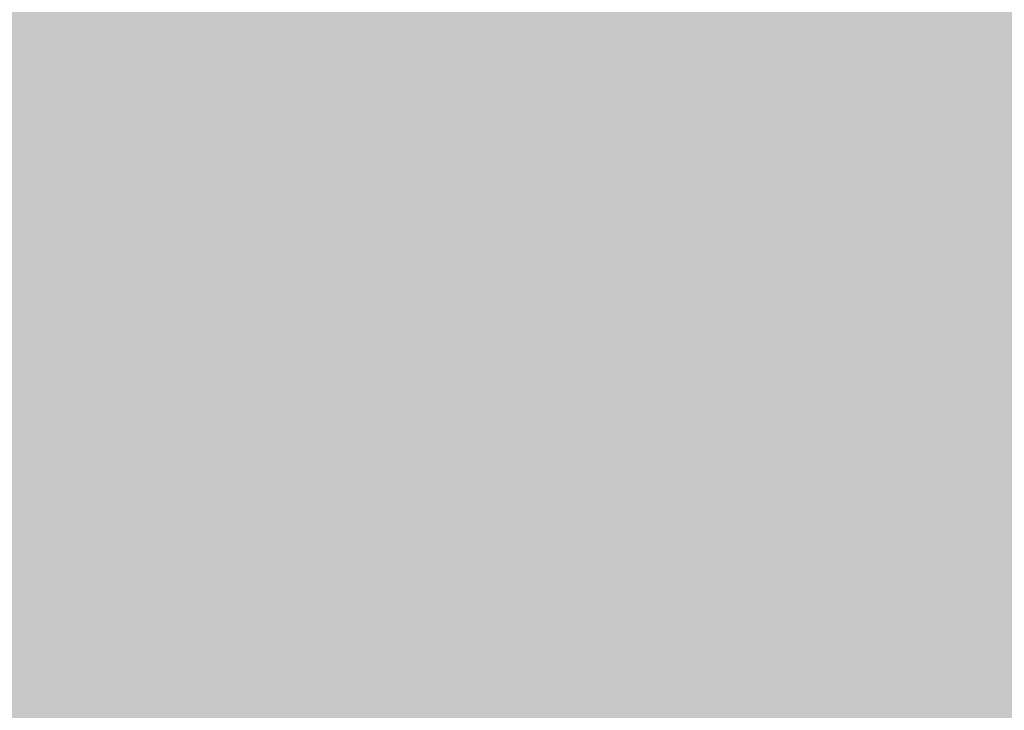
# Model space of a CAD drawing. Units: inches. Extents: x 2091 to 2899, y 967 to 2217.
# Tile 179 of 256: x 2203.151632 to 2203.161218, y 1152.253784 to 1152.260509. Entities that reach past the tile are written whole.
import ezdxf

# ---------------------------------------------------------------- set-up
doc = ezdxf.new("R2010")
doc.units = ezdxf.units.IN
doc.layers.add('A-WALL-PATT', color=141, linetype='Continuous', lineweight=13, true_color=0xadddf7)

msp = doc.modelspace()

# ---------------------------------------------------------------- hatches: boundary and pattern name
at = {"layer": 'A-WALL-PATT'}
h = msp.add_hatch(color=256, dxfattribs=at)
h.dxf.hatch_style = 1
h.paths.add_polyline_path([(2803.1436027, 2050.9190588), (2203.1436027, 2050.9190588), (2203.1436027, 1090.9190588), (2803.1436027, 1090.9190588)])
h.paths.add_polyline_path([(2635.7988501, 1147.5404649), (2674.5240524, 1147.5404649, 0.376086), (2678.5296653, 1152.8802017), (2678.5296653, 1159.5564734, 0.333335), (2674.524319, 1163.561846), (2674.524319, 1163.5618504), (2674.524319, 1192.9343904), (2635.8059707, 1192.9343904), (2597.0876225, 1192.9343904), (2597.0876225, 1163.561846, 0.333335), (2593.0822761, 1159.5564734), (2593.0822761, 1152.8802017, 0.376086), (2597.087889, 1147.5404649)], flags=0)
h.paths.add_polyline_path([(2436.0104329, 1278.2407784, 0.000483), (2435.9526433, 1278.215027, -0.001328), (2435.9356253, 1278.1116934, -0.001711), (2436.1164401, 1278.0407583, 0.002185)], flags=0)
h.paths.add_polyline_path([(2794.1436027, 1143.4190588), (2794.1436027, 1347.4190588), (2543.3701706, 1347.4190588), (2543.3701706, 1351.9190588), (2794.1436027, 1351.9190588), (2794.1436027, 1392.7135549), (2793.9473982, 1392.7135549), (2793.9473982, 1473.5368999), (2794.1436027, 1473.5368999), (2794.1436027, 1531.9190588), (2650.1436027, 1531.9190588), (2650.1436027, 1536.4190588), (2794.1436027, 1536.4190588), (2794.1436027, 1692.4190588), (2609.3756095, 1692.4190588), (2609.3756095, 1644.4190588), (2604.8756095, 1644.4190588), (2604.8756095, 1744.9190588), (2609.3756095, 1744.9190588), (2609.3756095, 1696.9190588), (2794.1436027, 1696.9190588), (2794.1436027, 1780.9190588), (2609.6436027, 1780.9190588), (2493.8756095, 1780.9190588), (2493.8756095, 1785.4190588), (2609.6436027, 1785.4190588), (2794.1436027, 1785.4190588), (2794.1436027, 1847.9388214), (2793.9512217, 1847.9388214), (2793.9512217, 1928.7621663), (2794.1436027, 1928.7621663), (2794.1436027, 1941.4190588), (2614.1436027, 1941.4190588), (2614.1436027, 1821.4190588), (2609.6436027, 1821.4190588), (2609.6436027, 1941.4190588), (2392.1436027, 1941.4190588), (2392.1436027, 1819.9190588), (2387.6436027, 1819.9190588), (2387.6436027, 1941.4190588), (2212.1436027, 1941.4190588), (2212.1436027, 1783.9190588), (2392.1436027, 1783.9190588), (2392.1436027, 1780.9190588), (2212.1436027, 1780.9190588), (2212.1436027, 1629.4190588), (2387.6436027, 1629.4190588), (2387.6436027, 1744.9190588), (2392.1436027, 1744.9190588), (2392.1436027, 1627.9190588), (2317.1436027, 1627.9190588), (2317.1436027, 1551.4190588), (2317.1436027, 1536.4190588), (2459.3835909, 1536.4190588), (2459.3835909, 1602.3964802), (2463.8835909, 1602.3964802), (2463.8835909, 1531.9190588), (2456.6436027, 1531.9190588), (2456.6436027, 1529.9190588), (2452.1436027, 1529.9190588), (2452.1436027, 1531.9190588), (2312.6436027, 1531.9190588), (2312.6436027, 1551.4190588), (2306.1436027, 1551.4190588), (2306.1436027, 1555.9190588), (2308.1436027, 1555.9190588), (2308.1436027, 1551.4190588), (2312.6436027, 1551.4190588), (2312.6436027, 1627.9190588), (2212.1436027, 1627.9190588), (2212.1436027, 1555.9190588), (2270.1436027, 1555.9190588), (2270.1436027, 1551.4190588), (2212.1436027, 1551.4190588), (2212.1436027, 1351.9190588), (2272.1436027, 1351.9190588), (2272.1436027, 1347.4190588), (2212.1436027, 1347.4190588), (2212.1436027, 1275.4190588), (2308.1436027, 1275.4190588), (2308.1436027, 1351.9190588), (2452.1436027, 1351.9190588), (2452.1436027, 1493.9190588), (2456.6436027, 1493.9190588), (2456.6436027, 1347.4190588), (2312.6436027, 1347.4190588), (2312.6436027, 1270.9190588), (2212.1436027, 1270.9190588), (2212.1436027, 1099.9190588), (2281.2375229, 1099.9190588), (2282.8710413, 1110.9138034), (2282.0083413, 1116.9966034), (2278.5577413, 1121.4204034), (2268.2056413, 1128.0562034), (2272.0876413, 1128.0562034), (2273.8129413, 1131.9270034), (2279.4203413, 1134.6919034), (2285.0278413, 1135.2449034), (2287.6158413, 1137.4568034), (2288.0471413, 1138.0098034), (2289.3411413, 1140.7747034), (2291.0665413, 1139.6687034), (2292.3605413, 1135.2449034), (2295.3798413, 1136.9038034), (2296.2425413, 1135.7979034), (2297.1052413, 1133.0330034), (2300.1246413, 1138.0098034), (2303.1439413, 1138.0098034), (2304.4379413, 1135.7979034), (2303.1439413, 1133.5860034), (2306.5946413, 1134.6919034), (2307.8887413, 1133.0330034), (2310.9080413, 1135.2449034), (2313.9274413, 1134.1389034), (2315.6268599, 1132.4271023), (2308.3200413, 1117.5496034), (2290.2038413, 1109.8079034), (2288.9098413, 1103.1721034), (2289.2723086, 1099.9190588), (2434.9182274, 1099.9190588), (2431.5932274, 1124.7880588), (2429.9302274, 1169.5530588), (2430.9271848, 1240.5196942), (2435.6589255, 1238.1861258), (2437.1352274, 1196.5540588), (2438.7982274, 1143.9730588), (2442.6782274, 1111.9980588), (2446.5582274, 1099.9190588), (2794.1436027, 1099.9190588), (2794.1436027, 1138.9190588), (2548.0324471, 1138.9190588), (2548.0324471, 1143.4190588), (2548.0324471, 1148.8190588), (2546.6684571, 1148.0315588), (2528.6856919, 1179.1786218, 0.256256), (2512.0324471, 1148.8190588), (2512.0324471, 1143.4190588), (2512.0324471, 1138.9190588), (2507.5324471, 1138.9190588), (2507.5324471, 1143.4190588), (2507.5324471, 1148.8190588, 0.256256), (2490.8792023, 1179.1786218), (2472.8964371, 1148.0315588), (2471.5324471, 1148.8190588), (2471.5324471, 1143.4190588), (2467.0324471, 1143.4190588), (2467.0324471, 1269.9457858, 0.039061), (2460.9099871, 1273.5800588), (2467.0324471, 1273.5800588), (2467.0324471, 1286.3253638, 0.014511), (2465.2161944, 1286.7619052), (2467.0324471, 1287.0525761), (2467.0324471, 1323.4190588), (2471.5324471, 1323.4190588), (2471.5324471, 1148.8190588), (2489.5324471, 1179.9959734), (2490.8964371, 1179.2084734), (2490.8792023, 1179.1786218, -0.256256), (2507.5324471, 1148.8190588), (2507.5324471, 1143.4190588), (2512.0324471, 1143.4190588), (2512.0324471, 1148.8190588, -0.256256), (2528.6856919, 1179.1786218), (2528.6684571, 1179.2084734), (2530.0324471, 1179.9959734), (2548.0324471, 1148.8190588), (2548.0324471, 1143.4190588)], flags=16)
h.paths.add_polyline_path([(2607.7685461, 1200.9450832), (2607.7685461, 1265.0306251), (2597.0876225, 1281.0520106), (2619.7845852, 1281.0520106), (2627.795278, 1337.1268598), (2635.7988501, 1337.1268598), (2643.8166634, 1337.1268598), (2651.8273562, 1281.0520106), (2674.524319, 1281.0520106), (2663.8433953, 1265.0306251), (2663.8433953, 1200.9450832), (2635.8059707, 1200.9450832)], flags=0)
edge = h.paths.add_edge_path(flags=0)
edge.add_ellipse((13303.8962153, 1272.9987247), major_axis=(-10595.3130399, 0.0000005), ratio=0.842303870086, start_angle=0.62823721906, end_angle=0.64655409989, ccw=False)
edge.add_ellipse((2711.7004495, 1156.8526781), major_axis=(2.2197691, 0), ratio=0.84230387, start_angle=111.5352435, end_angle=180.6282372, ccw=False)
edge.add_ellipse((13303.1562922, 1272.9987246), major_axis=(-10593.0263064, 0), ratio=0.842303869544, start_angle=0.52827147182, end_angle=0.64655409706, ccw=False)
edge.add_line((2710.7645961, 1175.3332951), (2710.1299858, 1175.3332951))
edge.add_ellipse((2710.1299858, 1176.5797752), major_axis=(1.4798461, 0), ratio=0.84230387, start_angle=180, end_angle=270, ccw=False)
edge.add_line((2708.6501397, 1176.5797752), (2708.6501397, 1200.7829144))
edge.add_ellipse((2710.1299858, 1200.7829144), major_axis=(1.4798461, 0), ratio=0.84230387, start_angle=90, end_angle=180, ccw=False)
edge.add_line((2710.1299858, 1202.0293944), (2710.4650752, 1202.0293944))
edge.add_ellipse((13303.1562922, 1272.9987246), major_axis=(-10593.0263064, 0), ratio=0.842303869544, start_angle=-0.09022908859, end_angle=0.38386677879, ccw=False)
edge.add_ellipse((2710.1299858, 1290.9270308), major_axis=(-1.4798461, 0), ratio=0.84230387, start_angle=0, end_angle=90, ccw=False)
edge.add_line((2708.6501397, 1290.9270308), (2708.6501397, 1315.13017))
edge.add_ellipse((2710.1299858, 1315.13017), major_axis=(-1.4798461, 0), ratio=0.84230387, start_angle=-90, end_angle=0, ccw=False)
edge.add_line((2710.1299858, 1316.3766501), (2710.7063141, 1316.3766501))
edge.add_ellipse((3238.4017202, 1296.2895655), major_axis=(528.2339998, 0), ratio=0.84230386954, start_angle=176.349572414, end_angle=177.820049686, ccw=False)
edge.add_ellipse((2775.0630432, 1071.4506962), major_axis=(313.3077613, 0), ratio=0.84230386954, start_angle=102.125965552, end_angle=103.780528989, ccw=False)
edge.add_ellipse((2775.0630432, 1078.3056979), major_axis=(-305.3028915, 0), ratio=0.84230386955, start_angle=-79.790461003, end_angle=-77.555372706, ccw=False)
edge.add_ellipse((2695.1417666, 1541.9753825), major_axis=(-250.9602162, 0), ratio=0.84230386954, start_angle=99.256566007, end_angle=102.554932644)
edge.add_line((2741.4103262, 1334.2142554), (2747.1325454, 1337.3784768))
edge.add_ellipse((2747.5386163, 1336.8574776), major_axis=(-0.739923, 0), ratio=0.84230387, start_angle=270, end_angle=307.9331305, ccw=False)
edge.add_ellipse((2747.5386163, 1336.8574776), major_axis=(-0.739923, 0), ratio=0.84230387, start_angle=232.0668695, end_angle=270, ccw=False)
edge.add_line((2747.9446872, 1337.3784768), (2753.6669064, 1334.2142554))
edge.add_ellipse((2799.935466, 1541.9753825), major_axis=(250.9602162, 0), ratio=0.84230386954, start_angle=257.445067356, end_angle=260.743433993)
edge.add_ellipse((2720.0141894, 1078.3056979), major_axis=(305.3028915, 0), ratio=0.84230386954, start_angle=77.555372707, end_angle=79.790461003, ccw=False)
edge.add_ellipse((2720.0141894, 1071.4506962), major_axis=(-313.3077613, 0), ratio=0.84230386954, start_angle=256.219471011, end_angle=257.874034448, ccw=False)
edge.add_ellipse((2256.6755124, 1296.2895655), major_axis=(-528.2339998, 0), ratio=0.84230386954, start_angle=182.179950314, end_angle=183.650427586, ccw=False)
edge.add_line((2784.3709184, 1316.3766501), (2784.9472468, 1316.3766501))
edge.add_ellipse((2784.9472468, 1315.13017), major_axis=(1.4798461, 0), ratio=0.84230387, start_angle=0, end_angle=90, ccw=False)
edge.add_line((2786.4270928, 1315.13017), (2786.4270928, 1290.9270308))
edge.add_ellipse((2784.9472468, 1290.9270308), major_axis=(1.4798461, 0), ratio=0.84230387, start_angle=270, end_angle=360, ccw=False)
edge.add_ellipse((-7808.0790596, 1272.9987246), major_axis=(10593.0263063, 0), ratio=0.842303869544, start_angle=-0.38386677879, end_angle=0.09022908859, ccw=False)
edge.add_line((2784.6121574, 1202.0293944), (2784.9472468, 1202.0293944))
edge.add_ellipse((2784.9472468, 1200.7829144), major_axis=(1.4798461, 0), ratio=0.84230387, start_angle=0, end_angle=90, ccw=False)
edge.add_line((2786.4270928, 1200.7829144), (2786.4270928, 1176.5797752))
edge.add_ellipse((2784.9472468, 1176.5797752), major_axis=(-1.4798461, 0), ratio=0.84230387, start_angle=90, end_angle=180, ccw=False)
edge.add_line((2784.9472468, 1175.3332951), (2784.3126365, 1175.3332951))
edge.add_ellipse((-7808.0790596, 1272.9987246), major_axis=(10593.0263063, 0), ratio=0.842303869544, start_angle=-0.61864319632, end_angle=-0.52827147182, ccw=False)
edge.add_ellipse((2783.3767831, 1156.8526781), major_axis=(-2.2197691, 0), ratio=0.84230387, start_angle=179.3717628, end_angle=248.4647566, ccw=False)
edge.add_ellipse((-7808.8189826, 1272.9987246), major_axis=(-10595.3130398, 0.0000036), ratio=0.842303865762, start_angle=179.3534459226, end_angle=179.37176280343, ccw=False)
edge.add_ellipse((2780.2973026, 1153.500793), major_axis=(-5.2464256, 0), ratio=0.84230387, start_angle=90, end_angle=179.3534459, ccw=False)
edge.add_line((2780.2973026, 1149.0817084), (2714.77993, 1149.0817084))
edge.add_ellipse((2714.77993, 1153.500793), major_axis=(5.2464256, 0), ratio=0.84230387, start_angle=180.6465541, end_angle=270, ccw=False)
edge = h.paths.add_edge_path(flags=0)
edge.add_line((2718.1873674, 1151.0078329), (2718.1873674, 1170.4723638))
edge.add_ellipse((2721.1470595, 1170.4723638), major_axis=(-2.9596921, 0), ratio=0.84230387, start_angle=-90, end_angle=0, ccw=False)
edge.add_line((2721.1470595, 1172.965324), (2773.9301731, 1172.965324))
edge.add_ellipse((2773.9301731, 1170.4723638), major_axis=(-2.9596921, 0), ratio=0.84230387, start_angle=180, end_angle=270, ccw=False)
edge.add_line((2776.8898652, 1170.4723638), (2776.8898652, 1151.0078329))
edge.add_line((2776.8898652, 1151.0078329), (2718.1873674, 1151.0078329))
edge = h.paths.add_edge_path(flags=0)
edge.add_line((2718.1873674, 1180.2341502), (2718.1873674, 1199.0578342))
edge.add_ellipse((2747.5386163, 1320.3986402), major_axis=(147.0179239, 0), ratio=0.84230386954, start_angle=256.40186531, end_angle=283.59813469)
edge.add_line((2776.8898652, 1199.0578342), (2776.8898652, 1180.2341502))
edge.add_ellipse((2747.5386163, 1301.5749562), major_axis=(147.0179239, 0), ratio=0.84230386954, start_angle=256.40186531, end_angle=283.59813469, ccw=False)
edge = h.paths.add_edge_path(flags=0)
edge.add_ellipse((13303.1562922, 1272.9987246), major_axis=(-10591.5464603, 0), ratio=0.842303869555, start_angle=0.05559431352, end_angle=0.37776419393, ccw=False)
edge.add_line((2711.6168595, 1262.7217103), (2715.6674076, 1249.4953957))
edge.add_ellipse((6413.8919626, 1241.691919), major_axis=(-3698.2361592, 0), ratio=0.842303869547, start_angle=-0.120897369, end_angle=0.3640763489)
edge.add_line((2715.7610383, 1218.1924547), (2711.9343065, 1203.167361))
edge = h.paths.add_edge_path(flags=0)
edge.add_line((2718.1873674, 1251.074566), (2716.0024854, 1267.4504351))
edge.add_ellipse((2742.1511746, 1202.1895399), major_axis=(81.7725845, 0), ratio=0.8423038695, start_angle=94.277420963, end_angle=111.834953797, ccw=False)
edge.add_line((2737.0097482, 1270.9306255), (2758.0674844, 1270.9306255))
edge.add_ellipse((2752.926058, 1202.1895399), major_axis=(81.7725845, 0), ratio=0.8423038695, start_angle=68.165046203, end_angle=85.722579037, ccw=False)
edge.add_line((2779.0747472, 1267.4504351), (2776.8898652, 1251.074566))
edge.add_ellipse((2750.3380588, 1187.8853558), major_axis=(79.5796641, 0), ratio=0.8423038695, start_angle=67.208085122, end_angle=85.129930403)
edge.add_line((2756.0346562, 1254.7436557), (2739.0425764, 1254.7436557))
edge.add_ellipse((2744.7391738, 1187.8853558), major_axis=(79.5796641, 0), ratio=0.8423038695, start_angle=94.870069597, end_angle=112.791914878)
edge = h.paths.add_edge_path(flags=0)
edge.add_line((2783.1429261, 1203.167361), (2779.3161943, 1218.1924547))
edge.add_ellipse((-918.81473, 1241.691919), major_axis=(3698.2361592, 0), ratio=0.842303869546, start_angle=-0.3640763489, end_angle=0.120897369)
edge.add_line((2779.409825, 1249.4953957), (2783.4603731, 1262.7217103))
edge.add_ellipse((-7808.0790596, 1272.9987246), major_axis=(-10591.5464603, 0), ratio=0.84230386954, start_angle=179.6222358061, end_angle=179.94440568651, ccw=False)
edge = h.paths.add_edge_path(flags=0)
edge.add_ellipse((2734.2008921, 1286.6904402), major_axis=(-0.3566086, 6.3400775), ratio=0.603833576, start_angle=89.00201428, end_angle=253.65740805, ccw=False)
edge.add_line((2730.3690013, 1286.5418057), (2730.3690013, 1301.3519803))
edge.add_line((2730.3690013, 1301.3519803), (2735.9133107, 1305.2148028))
edge.add_ellipse((2736.3849168, 1304.7345612), major_axis=(0.739923, 0), ratio=0.84230387, start_angle=90, end_angle=134.4802109, ccw=False)
edge.add_line((2736.3849168, 1305.3578013), (2738.0327829, 1305.3578013))
edge.add_line((2738.0327829, 1305.3578013), (2738.0327829, 1307.7079274))
edge.add_ellipse((2794.201642, 1307.7079274), major_axis=(56.168859, 0), ratio=0.8423038695, start_angle=150.5614304, end_angle=180, ccw=False)
edge.add_ellipse((2700.8755906, 1307.7079274), major_axis=(-56.168859, 0), ratio=0.8423038695, start_angle=180, end_angle=209.4385696, ccw=False)
edge.add_line((2757.0444497, 1307.7079274), (2757.0444497, 1305.3578013))
edge.add_line((2757.0444497, 1305.3578013), (2758.6923157, 1305.3578013))
edge.add_ellipse((2758.6923157, 1304.7345612), major_axis=(-0.739923, 0), ratio=0.84230387, start_angle=225.5197891, end_angle=270, ccw=False)
edge.add_line((2759.1639219, 1305.2148028), (2764.7082312, 1301.3519803))
edge.add_line((2764.7082312, 1301.3519803), (2764.7082312, 1286.5418057))
edge.add_ellipse((2760.8763405, 1286.6904402), major_axis=(0.3566086, 6.3400775), ratio=0.603833576, start_angle=106.34259195, end_angle=270.99798572, ccw=False)
edge.add_line((2757.0444497, 1285.7970896), (2757.0444497, 1307.7079274))
edge.add_ellipse((2700.8755906, 1307.7079274), major_axis=(-56.168859, 0), ratio=0.8423038695, start_angle=180, end_angle=209.4385696)
edge.add_ellipse((2794.201642, 1307.7079274), major_axis=(56.168859, 0), ratio=0.8423038695, start_angle=150.5614304, end_angle=180)
edge.add_line((2738.0327829, 1307.7079274), (2738.0327829, 1285.7970896))
h.paths.add_polyline_path([(2417.8122727, 1104.449704), (2413.4922727, 1102.529704), (2410.6122727, 1103.969704), (2409.1722727, 1106.369704), (2407.2522727, 1107.329704), (2406.2922727, 1109.729704), (2405.3322727, 1114.049704), (2405.3322727, 1117.889704), (2406.2922727, 1120.129704), (2407.2522727, 1119.809704), (2408.8483218, 1118.3276585), (2410.1739451, 1119.4241703), (2410.2112727, 1120.405704), (2411.0407305, 1121.4190541), (2410.6992727, 1119.858704), (2410.1739451, 1119.4241703), (2410.0884515, 1117.1761095), (2411.1328361, 1116.2063237), (2413.9722727, 1119.329704), (2416.8522727, 1120.769704), (2416.8697209, 1120.7987842), (2417.0350713, 1119.4051162), (2417.8962134, 1118.1433844), (2418.2922727, 1118.369704), (2419.5444467, 1120.0392692), (2419.3609153, 1118.387487), (2419.0321078, 1119.3561507), (2418.3989394, 1118.5119262), (2419.2522727, 1114.529704), (2418.7940909, 1107.1987949)], flags=0)
h.paths.add_polyline_path([(2508.8701706, 1347.4190588), (2508.3701706, 1347.4190588), (2508.3701706, 1351.9190588), (2508.8701706, 1351.9190588)], flags=0)
h.paths.add_polyline_path([(2473.3701706, 1347.4190588), (2472.3701706, 1347.4190588), (2467.8701706, 1347.4190588), (2467.8701706, 1455.4190588), (2472.3701706, 1455.4190588), (2472.3701706, 1352.4190588), (2473.3701706, 1352.4190588)], flags=0)
h.paths.add_polyline_path([(2352.106244, 1217.4461971), (2349.226244, 1218.8861971), (2347.786244, 1221.2861971), (2345.866244, 1222.2461971), (2344.906244, 1224.6461971), (2343.946244, 1228.9661971), (2343.946244, 1232.8061971), (2344.906244, 1235.0461971), (2345.866244, 1234.7261971), (2347.4622931, 1233.2441515), (2348.7879164, 1234.3406634), (2348.825244, 1235.3221971), (2349.6547018, 1236.3355471), (2349.313244, 1234.7751971), (2348.7879164, 1234.3406634), (2348.7024228, 1232.0926025), (2349.7468074, 1231.1228168), (2352.586244, 1234.2461971), (2355.466244, 1235.6861971), (2355.4836921, 1235.7152773), (2355.6490426, 1234.3216093), (2356.5101846, 1233.0598774), (2356.906244, 1233.2861971), (2358.1584179, 1234.9557623), (2357.9748866, 1233.3039801), (2357.6460791, 1234.2726438), (2357.0129107, 1233.4284193), (2357.866244, 1229.4461971), (2357.4080622, 1222.115288), (2356.426244, 1219.3661971)], flags=0)
h.paths.add_polyline_path([(2348.2967999, 1112.2244204), (2347.0137999, 1112.3104204), (2345.5297999, 1114.1274204), (2345.7317999, 1115.8584204), (2346.8117999, 1116.9824204), (2346.8117999, 1114.6464204), (2345.8667999, 1114.2144204), (2346.8797999, 1114.3004204)], flags=0)
h.paths.add_polyline_path([(2347.0137999, 1110.9264204), (2346.2717999, 1110.4934204), (2346.6097999, 1111.1864204)], flags=0)
h.paths.add_polyline_path([(2345.8667999, 1118.1944204), (2345.5297999, 1117.3294204), (2343.7077999, 1118.0214204), (2344.3827999, 1118.6264204)], flags=0)
h.paths.add_polyline_path([(2346.6767999, 1109.2824204), (2346.0697999, 1108.0714204), (2345.8667999, 1110.0614204)], flags=0)
h.paths.add_polyline_path([(2345.0567999, 1119.7514204), (2343.6397999, 1119.7514204), (2343.9777999, 1121.1354204)], flags=0)
h.paths.add_polyline_path([(2345.2597999, 1116.5504204), (2345.1247999, 1115.8584204), (2344.9217999, 1115.6854204), (2344.7197999, 1116.3774204)], flags=0)
h.paths.add_polyline_path([(2345.6647999, 1112.3104204), (2345.4617999, 1111.5324204), (2344.0447999, 1111.9644204), (2344.6517999, 1112.5704204)], flags=0)
h.paths.add_polyline_path([(2345.1917999, 1113.3494204), (2344.4497999, 1113.8684204), (2344.7197999, 1114.3874204)], flags=0)
h.paths.add_polyline_path([(2344.6517999, 1116.8094204), (2344.1797999, 1115.6854204), (2344.6517999, 1115.3394204), (2343.9097999, 1114.9064204), (2343.0327999, 1115.9444204), (2343.6397999, 1116.4634204)], flags=0)
h.paths.add_polyline_path([(2345.8667999, 1106.6864204), (2344.9897999, 1105.5624204), (2344.5167999, 1106.6004204)], flags=0)
h.paths.add_polyline_path([(2344.8547999, 1110.0614204), (2344.5167999, 1109.2824204), (2344.1127999, 1109.7154204)], flags=0)
h.paths.add_polyline_path([(2344.0447999, 1113.5224204), (2343.4377999, 1113.0894204), (2342.7627999, 1113.9544204)], flags=0)
h.paths.add_polyline_path([(2344.3147999, 1111.0124204), (2342.9647999, 1110.3204204), (2342.9647999, 1111.0994204)], flags=0)
h.paths.add_polyline_path([(2345.1247999, 1104.6974204), (2344.5847999, 1103.7454204), (2344.4497999, 1104.2644204)], flags=0)
h.paths.add_polyline_path([(2342.8297999, 1121.2224204), (2341.7497999, 1120.5304204), (2340.5357999, 1121.0494204), (2340.1307999, 1121.8284204), (2340.6707999, 1122.9524204), (2341.1427999, 1121.8284204), (2341.6147999, 1122.0014204)], flags=0)
h.paths.add_polyline_path([(2342.9647999, 1119.7514204), (2343.0327999, 1118.4534204), (2342.0877999, 1118.0214204), (2342.0197999, 1119.4914204)], flags=0)
h.paths.add_polyline_path([(2342.6947999, 1116.8964204), (2341.9527999, 1116.6364204), (2342.0197999, 1117.3294204)], flags=0)
h.paths.add_polyline_path([(2343.0327999, 1112.2244204), (2342.0197999, 1111.7914204), (2341.5477999, 1112.2244204), (2342.3577999, 1113.3494204)], flags=0)
h.paths.add_polyline_path([(2343.7747999, 1104.4374204), (2342.6277999, 1102.8804204), (2342.6947999, 1104.6104204), (2343.4377999, 1105.1294204)], flags=0)
h.paths.add_polyline_path([(2342.0197999, 1115.0794204), (2340.8057999, 1115.5124204), (2340.9407999, 1116.3774204)], flags=0)
h.paths.add_polyline_path([(2341.4807999, 1120.0974204), (2341.4807999, 1119.4054204), (2341.0757999, 1119.5784204), (2341.1427999, 1120.0974204)], flags=0)
h.paths.add_polyline_path([(2341.8177999, 1114.4734204), (2340.9407999, 1113.0894204), (2340.8057999, 1114.5604204)], flags=0)
h.paths.add_polyline_path([(2341.1427999, 1118.5404204), (2340.9407999, 1116.9824204), (2339.0507999, 1117.6754204), (2339.0507999, 1118.6264204)], flags=0)
h.paths.add_polyline_path([(2342.6947999, 1101.6684204), (2341.9527999, 1101.8414204), (2342.5597999, 1102.3614204)], flags=0)
h.paths.add_polyline_path([(2340.3327999, 1119.6654204), (2338.4437999, 1119.5784204), (2337.9037999, 1120.3574204), (2339.6577999, 1120.6164204)], flags=0)
h.paths.add_polyline_path([(2340.3327999, 1115.3394204), (2340.0627999, 1113.6954204), (2339.3877999, 1115.3394204)], flags=0)
h.paths.add_polyline_path([(2341.8177999, 1103.8314204), (2341.5477999, 1102.8804204), (2341.1427999, 1103.6584204)], flags=0)
h.paths.add_polyline_path([(2339.0507999, 1122.8664204), (2337.2957999, 1121.8284204), (2337.0937999, 1123.1254204), (2337.7687999, 1123.8184204)], flags=0)
h.paths.add_polyline_path([(2339.1177999, 1121.7414204), (2338.8477999, 1121.2224204), (2338.1737999, 1121.0494204), (2338.3757999, 1121.5684204)], flags=0)
h.paths.add_polyline_path([(2339.1857999, 1119.3194204), (2338.6457999, 1118.7134204), (2338.2407999, 1118.1074204), (2338.2407999, 1118.8864204)], flags=0)
h.paths.add_polyline_path([(2341.1427999, 1101.9284204), (2340.6027999, 1101.2364204), (2340.0627999, 1101.8414204), (2340.6027999, 1102.3614204)], flags=0)
h.paths.add_polyline_path([(2337.6337999, 1117.7614204), (2336.6207999, 1118.2804204), (2337.2957999, 1118.9724204)], flags=0)
h.paths.add_polyline_path([(2336.8237999, 1119.5784204), (2334.7987999, 1118.9724204), (2335.2037999, 1120.3574204), (2336.5537999, 1120.8764204)], flags=0)
h.paths.add_polyline_path([(2339.1177999, 1100.4574204), (2337.3637999, 1100.5434204), (2336.7557999, 1101.2364204)], flags=0)
h.paths.add_polyline_path([(2336.3507999, 1122.4334204), (2336.0137999, 1121.9144204), (2334.9337999, 1122.4334204), (2334.5287999, 1123.4714204), (2335.7437999, 1122.7794204)], flags=0)
h.paths.add_polyline_path([(2334.7317999, 1120.8764204), (2334.2587999, 1120.3574204), (2334.0567999, 1120.7894204), (2334.5967999, 1121.3084204)], flags=0)
h.paths.add_polyline_path([(2334.4617999, 1122.1744204), (2332.5717999, 1121.3084204), (2331.3567999, 1122.1744204), (2332.0997999, 1122.8664204)], flags=0)
h.paths.add_polyline_path([(2334.2587999, 1118.5404204), (2333.3817999, 1118.4534204), (2333.6517999, 1119.3194204)], flags=0)
h.paths.add_polyline_path([(2335.5417999, 1102.2744204), (2334.1917999, 1102.6204204), (2335.2717999, 1103.3124204)], flags=0)
h.paths.add_polyline_path([(2332.7067999, 1119.6654204), (2331.6947999, 1120.4434204), (2332.5047999, 1120.7894204)], flags=0)
h.paths.add_polyline_path([(2334.7317999, 1101.1494204), (2333.5167999, 1101.5824204), (2333.9887999, 1101.7554204)], flags=0)
h.paths.add_polyline_path([(2332.6397999, 1116.6364204), (2331.0867999, 1116.2904204), (2331.9647999, 1118.1944204)], flags=0)
h.paths.add_polyline_path([(2330.7497999, 1121.5684204), (2330.2767999, 1120.2704204), (2328.5227999, 1119.3194204), (2328.9947999, 1121.0494204)], flags=0)
h.paths.add_polyline_path([(2330.7497999, 1118.6264204), (2330.0077999, 1117.5024204), (2329.8727999, 1118.0214204)], flags=0)
h.paths.add_polyline_path([(2332.0997999, 1102.3614204), (2330.5467999, 1102.0144204), (2331.6947999, 1102.9664204)], flags=0)
h.paths.add_polyline_path([(2329.5347999, 1113.6084204), (2329.0627999, 1112.3104204), (2328.5897999, 1113.3494204)], flags=0)
h.paths.add_polyline_path([(2328.3877999, 1117.8484204), (2327.5097999, 1116.5504204), (2327.1727999, 1117.7614204)], flags=0)
h.paths.add_polyline_path([(2329.7377999, 1106.5134204), (2329.5347999, 1105.3024204), (2328.2527999, 1106.0814204)], flags=0)
h.paths.add_polyline_path([(2328.6577999, 1114.3874204), (2328.0497999, 1114.1274204), (2328.3197999, 1114.9064204)], flags=0)
h.paths.add_polyline_path([(2328.3197999, 1112.2244204), (2327.1057999, 1112.1374204), (2326.7007999, 1112.6564204)], flags=0)
h.paths.add_polyline_path([(2326.9027999, 1115.2524204), (2326.7007999, 1114.1274204), (2325.2157999, 1113.6084204), (2326.0927999, 1115.3394204)], flags=0)
h.paths.add_polyline_path([(2326.6327999, 1108.3304204), (2326.0927999, 1107.3794204), (2325.8907999, 1108.5034204), (2326.4977999, 1109.1094204)], flags=0)
h.paths.add_polyline_path([(2615.1436027, 1531.9190588), (2609.6436027, 1531.9190588), (2609.6436027, 1620.4190588), (2614.1436027, 1620.4190588), (2614.1436027, 1536.4190588), (2615.1436027, 1536.4190588)], flags=0)
h.paths.add_polyline_path([(2545.1436027, 1563.4190588), (2464.1436027, 1563.4190588), (2464.1436027, 1632.4190588), (2509.1436027, 1632.4190588), (2509.1436027, 1627.9190588), (2509.1436027, 1603.9190588), (2468.6436027, 1603.9190588), (2468.6436027, 1567.9190588), (2540.6436027, 1567.9190588), (2540.6436027, 1591.9190588), (2545.1436027, 1591.9190588)], flags=0)
h.paths.add_polyline_path([(2388.9690483, 1549.985735), (2357.4341811, 1549.985735), (2357.4341811, 1623.3607783), (2399.3627772, 1623.3607783), (2435.6894654, 1623.3607783), (2435.5925469, 1602.5592734), (2435.5925469, 1602.3964802), (2388.9690483, 1602.3964802)], flags=0)
h.paths.add_polyline_path([(2388.8806282, 1555.8091511), (2374.9044295, 1555.8091511), (2374.9044295, 1600.5715641), (2374.9044295, 1615.4576454), (2406.3508766, 1615.4576454), (2406.3508766, 1618.9394309), (2412.1742927, 1615.4576454), (2406.3508766, 1611.9758599), (2406.3508766, 1615.4576454), (2388.8806282, 1615.4576454)], flags=0)
h.paths.add_polyline_path([(2568.8756095, 1644.4190588), (2453.3756095, 1644.4190588), (2453.3756095, 1785.4190588), (2457.8756095, 1785.4190588), (2457.8756095, 1648.9190588), (2568.8756095, 1648.9190588)], flags=0)
h.paths.add_polyline_path([(2212.1436027, 1945.9190588), (2212.1436027, 2041.9190588), (2794.1436027, 2041.9190588), (2794.1436027, 1945.9190588)], flags=16)
h.paths.add_polyline_path([(2271.0827276, 1964.3172377), (2776.852968, 1964.3172377), (2776.852968, 2037.1696226), (2271.0827276, 2037.1696226)], flags=8)
h.paths.add_polyline_path([(2380.6492852, 1536.8241435), (2461.0408087, 1536.8241435), (2461.0408087, 1554.6525871), (2380.6492852, 1554.6525871)], flags=8)
h.paths.add_polyline_path([(2240.7557092, 1609.7254508), (2309.1858294, 1609.7254508), (2309.1858294, 1617.6982037), (2240.7557092, 1617.6982037)], flags=8)
h.paths.add_polyline_path([(2212.6772554, 1313.5041021), (2282.5915203, 1313.5041021), (2282.5915203, 1322.7452389), (2212.6772554, 1322.7452389)], flags=8)
h.paths.add_polyline_path([(2457.111976, 1114.778574), (2558.4815807, 1114.778574), (2558.4815807, 1142.2196823), (2457.111976, 1142.2196823)], flags=8)
h.paths.add_polyline_path([(2473.4423372, 1273.0100672), (2604.6412257, 1273.0100672), (2604.6412257, 1318.3469349), (2473.4423372, 1318.3469349)], flags=8)
h.paths.add_polyline_path([(2638.8763024, 1626.9774316), (2684.2503675, 1627.9767377), (2684.0384825, 1637.5974944), (2638.6644174, 1636.5981884)], flags=8)
h.paths.add_polyline_path([(2537.5905538, 1453.7934466), (2628.3895472, 1453.7934466), (2628.3895472, 1475.3448114), (2537.5905538, 1475.3448114)], flags=8)
h.paths.add_polyline_path([(2504.1376376, 1714.6323972), (2554.6471875, 1714.6323972), (2554.6471875, 1730.2377115), (2504.1376376, 1730.2377115)], flags=8)
h.paths.add_polyline_path([(2487.5011806, 1575.6518716), (2535.0971214, 1575.6518716), (2535.0971214, 1598.3776456), (2487.5011806, 1598.3776456)], flags=8)
h.paths.add_polyline_path([(2709.0994004, 1735.7102784), (2740.0166009, 1735.7102784), (2740.0166009, 1749.9376406), (2709.0994004, 1749.9376406)], flags=8)
h.paths.add_polyline_path([(2442.4384239, 1792.1716575), (2564.7288353, 1792.1716575), (2564.7288353, 1842.0001626), (2442.4384239, 1842.0001626)], flags=8)
h.paths.add_polyline_path([(2655.8158012, 1809.6440763), (2789.5201425, 1806.6937963), (2790.0849768, 1832.2916379), (2656.3806355, 1835.2419179)], flags=8)
h.paths.add_polyline_path([(2234.8426972, 1797.7201432), (2368.5928512, 1794.7688523), (2369.1607182, 1820.504132), (2235.4105642, 1823.4554229)], flags=8)
h.paths.add_polyline_path([(2245.1384659, 1644.0063348), (2398.4277329, 1640.6238997), (2398.9948417, 1666.3248199), (2245.7055747, 1669.7072549)], flags=8)
h.paths.add_polyline_path([(2306.1428474, 1431.1685186), (2413.7683138, 1428.7936873), (2414.3331481, 1454.3915289), (2306.7076817, 1456.7663602)], flags=8)
h.paths.add_polyline_path([(2306.834582, 1458.2331447), (2393.3804836, 1456.3234487), (2393.9328082, 1481.3543583), (2307.3869066, 1483.2640542)], flags=8)

doc.saveas('drawing.dxf')
